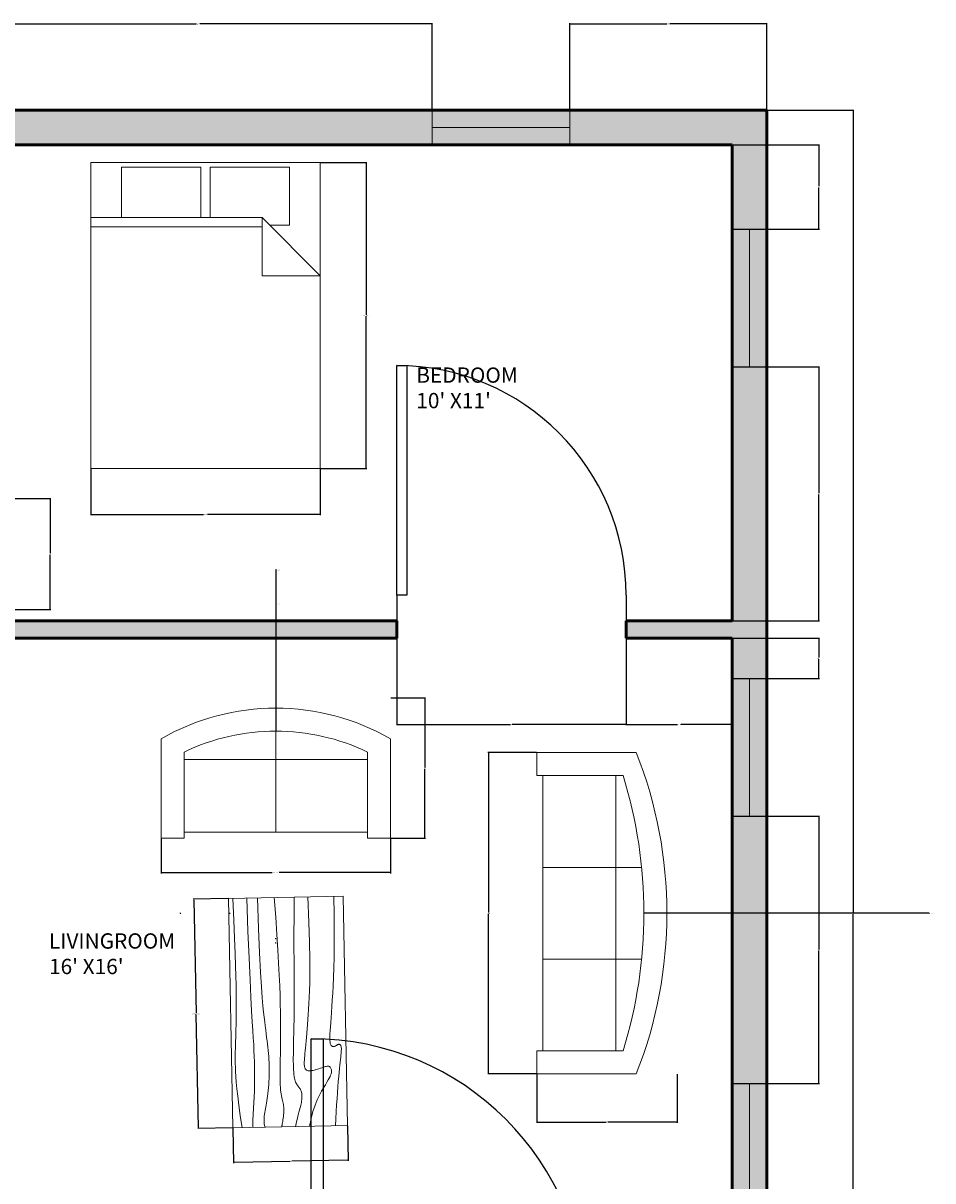
# Model space of a CAD drawing. Units: inches. Extents: x 7 to 493, y -11 to 454.
# Tile 4 of 4: x 255 to 493, y 152 to 454. Entities that reach past the tile are written whole.
import ezdxf

# ---------------------------------------------------------------- set-up
doc = ezdxf.new("R2010")
doc.units = ezdxf.units.IN
doc.header["$MEASUREMENT"] = 0
for name, color, linetype, lineweight in [('A-ANNO-DIMS', 2, 'Continuous', 18), ('A-AREA-IDEN', 7, 'Continuous', 25), ('A-WALL', 7, 'Continuous', 50), ('doors', 40, 'Continuous', 25), ('furniture', 220, 'Continuous', 18), ('window', 30, 'Continuous', 18)]:
    doc.layers.add(name, color=color, linetype=linetype, lineweight=lineweight)
doc.layers.add('A-WALL-PATT', color=251, linetype='Continuous', lineweight=13, true_color=0x636466)
doc.styles.get("Standard").update_dxf_attribs({"font": 'arial.ttf'})
doc.dimstyles.get("Standard").update_dxf_attribs({"dimtxt": 0.18, "dimasz": 0.18, "dimexe": 0.18, "dimexo": 0.0625, "dimgap": 0.09, "dimtad": 0, "dimtih": 1, "dimtoh": 1, "dimdec": 4, "dimzin": 0, "dimdsep": 46, "dimtxsty": 'Standard', "dimcen": 0.09, "dimadec": 0, "dimazin": 0, "dimtfac": 1, "dimtdec": 4, "dimtofl": 0, "dimtmove": 0, "dimatfit": 3, "dimfxl": 1, "dimtolj": 1, "dimtzin": 0, "dimarcsym": 0})

# ---------------------------------------------------------------- blocks, each defined once
blk = doc.blocks.new('Sofa - Roundback 7 ft.')
for p, q in [((-12.00002, -32.4421), (-12.00003, -6.5971)), ((11.99997, -32.4421), (11.99998, -6.5971)), ((-36.000027, -34), (-36.000027, -11.4696)), ((35.99998, -34), (35.99998, -11.4696)), ((-35.999844, -13.3819), (35.9998, -13.3819)), ((-36.000027, -32.4421), (35.99998, -32.4421))]:
    blk.add_line(p, q)
for points in [[(-36.000027, -34), (-42.000027, -34), (-42.000027, -8)], [(41.99998, -8), (41.99998, -34), (35.99998, -34)]]:
    blk.add_lwpolyline(points)
for centre, radius, start, end in [((0, -114.25), 114.25, 68.43141, 111.5686), ((-0.00001, -127.1968), 121.1968, 72.72033, 107.2797)]:
    blk.add_arc(centre, radius, start, end)
blk = doc.blocks.new('Sofa - Roundback Loveseat 5 ft.')
for p, q in [((0, -32.44198), (0, -5.99998)), ((-24, -33.99998), (-24, -11.46958)), ((24.00004, -33.99998), (24.00004, -11.46958)), ((-23.9998, -13.38178), (23.99986, -13.38178)), ((-24, -32.44198), (24.00004, -32.44198))]:
    blk.add_line(p, q)
for points in [[(-24, -33.99998), (-30, -33.99998), (-30, -7.99998)], [(30.00004, -7.99998), (30.00004, -33.99998), (24.00004, -33.99998)]]:
    blk.add_lwpolyline(points)
for centre, radius, start, end in [((0, -60.24998), 60.24998, 60.13715, 119.8628), ((0, -61.38438), 55.38444, 64.32083, 115.6792)]:
    blk.add_arc(centre, radius, start, end)
blk = doc.blocks.new('Bed - Queen')
for p, q in [((0, -80.00003), (0, 0)), ((0, 0), (59.99999, 0)), ((59.99999, 0), (59.99999, -80.00003)), ((7.99999, -1.2), (28.79998, -1.2)), ((7.99999, -14.4), (7.99999, -1.2)), ((28.79998, -1.2), (28.79998, -14.4)), ((31.19999, -1.2), (51.99999, -1.2)), ((31.19999, -14.4), (31.19999, -1.2)), ((51.99999, -1.2), (51.99999, -16.4)), ((0, -14.4), (44.8, -14.4)), ((59.99999, -29.6), (44.8, -14.4)), ((44.8, -14.4), (44.8, -29.6)), ((44.8, -16.8), (0, -16.8)), ((51.99999, -16.4), (46.79936, -16.4)), ((44.8, -29.6), (59.99999, -29.6)), ((59.99999, -80.00003), (0, -80.00003))]:
    blk.add_line(p, q)
blk = doc.blocks.new('Table - Rectangular Woodgrain 60 x 30 in.')
for p, q in [((0, 0), (0, -30)), ((60, 0), (0, 0)), ((60, -30), (60, 0)), ((0, -30), (60, -30))]:
    blk.add_line(p, q)
for points in [[(0, -2.4), (4.8155, -2.418), (9.0302, -2.4688), (12.709, -2.5477), (15.9167, -2.65), (18.7181, -2.7711), (21.1781, -2.9063), (23.3616, -3.0508), (25.3333, -3.2), (27.1477, -3.3495), (28.8172, -3.4958), (30.3437, -3.636), (31.7291, -3.7667), (32.9756, -3.8849), (34.0849, -3.9875), (35.059, -4.0714), (35.9, -4.1334), (36.6114, -4.1711), (37.2041, -4.1854), (37.6906, -4.1779), (38.0833, -4.15), (38.3948, -4.1034), (38.6375, -4.0396), (38.8239, -3.9602), (38.9666, -3.8667), (39.0764, -3.7608), (39.1573, -3.6448), (39.2116, -3.521), (39.2416, -3.3917), (39.2498, -3.2593), (39.2385, -3.1261), (39.21, -2.9944), (39.1666, -2.8667), (39.111, -2.7447), (39.0468, -2.6281), (38.978, -2.5163), (38.9083, -2.4083), (38.8418, -2.3035), (38.7823, -2.201), (38.7337, -2.1001), (38.7, -2), (38.6844, -1.9003), (38.6875, -1.8021), (38.7094, -1.707), (38.75, -1.6167), (38.8094, -1.5326), (38.8875, -1.4563), (38.9844, -1.3893), (39.1, -1.3333), (39.2351, -1.2896), (39.3937, -1.2583), (39.5804, -1.2396), (39.8, -1.2333), (40.057, -1.2396), (40.3562, -1.2583), (40.7023, -1.2896), (41.1, -1.3333), (41.5547, -1.3895), (42.0755, -1.4573), (42.6721, -1.5361), (43.3542, -1.625), (44.1316, -1.7233), (45.014, -1.8302), (46.0114, -1.9449), (47.1333, -2.0667), (48.3862, -2.1947), (49.7625, -2.3281), (51.2513, -2.4663), (52.8416, -2.6083), (54.5226, -2.7535), (56.2833, -2.9011), (58.1127, -3.0501), (60, -3.2)], [(0, -9.2), (6.5759, -9.0858), (11.9385, -9.0365), (16.2527, -9.0418), (19.6833, -9.0917), (22.3952, -9.1759), (24.5531, -9.2844), (26.322, -9.4069), (27.8666, -9.5333), (29.3241, -9.6553), (30.7203, -9.7719), (32.0532, -9.8837), (33.3208, -9.9917), (34.5213, -10.0965), (35.6526, -10.199), (36.7128, -10.2999), (37.7, -10.4), (38.6129, -10.4996), (39.4531, -10.5969), (40.223, -10.6895), (40.925, -10.775), (41.5613, -10.8512), (42.1344, -10.9156), (42.6465, -10.966), (43.1, -11), (43.4976, -11.0158), (43.8437, -11.0136), (44.143, -10.9942), (44.4, -10.9583), (44.6195, -10.9069), (44.8062, -10.8406), (44.9648, -10.7603), (45.1, -10.6667), (45.2155, -10.5598), (45.3114, -10.4365), (45.3871, -10.2929), (45.4416, -10.125), (45.4743, -9.929), (45.4844, -9.7011), (45.4709, -9.4371), (45.4333, -9.1333), (45.3716, -8.7883), (45.2896, -8.4104), (45.1919, -8.0107), (45.0833, -7.6), (44.9685, -7.1893), (44.8521, -6.7896), (44.7388, -6.4117), (44.6333, -6.0667), (44.54, -5.7628), (44.4614, -5.4979), (44.4001, -5.2675), (44.3583, -5.0667), (44.3384, -4.8909), (44.3427, -4.7354), (44.3736, -4.5956), (44.4333, -4.4667), (44.5236, -4.3453), (44.6427, -4.2333), (44.7884, -4.1339), (44.9583, -4.05), (45.1501, -3.9849), (45.3614, -3.9417), (45.59, -3.9234), (45.8333, -3.9333), (46.0915, -3.9749), (46.3734, -4.0531), (46.6906, -4.1736), (47.0542, -4.3417), (47.4756, -4.5629), (47.9661, -4.8427), (48.5372, -5.1866), (49.2, -5.6), (49.9676, -6.0844), (50.8594, -6.625), (51.8965, -7.2031), (53.1, -7.8), (54.491, -8.3969), (56.0906, -8.975), (57.9199, -9.5156), (60, -10)], [(0, -12.8), (5.1847, -12.9322), (9.6213, -13.0323), (13.3963, -13.1059), (16.5958, -13.1583), (19.3063, -13.1952), (21.614, -13.2219), (23.6054, -13.2439), (25.3666, -13.2667), (26.9728, -13.2947), (28.4531, -13.3281), (29.8256, -13.3663), (31.1083, -13.4083), (32.3191, -13.4535), (33.476, -13.501), (34.597, -13.5501), (35.7, -13.6), (36.7984, -13.6497), (37.8875, -13.6979), (38.9578, -13.743), (40, -13.7833), (41.0047, -13.8174), (41.9625, -13.8438), (42.864, -13.8607), (43.7, -13.8667), (44.4631, -13.8604), (45.1552, -13.8417), (45.7801, -13.8104), (46.3416, -13.7667), (46.8439, -13.7104), (47.2906, -13.6417), (47.6858, -13.5604), (48.0333, -13.4667), (48.3375, -13.3608), (48.6042, -13.2448), (48.8396, -13.121), (49.05, -12.9917), (49.2417, -12.8593), (49.4208, -12.7261), (49.5937, -12.5944), (49.7667, -12.4667), (49.9452, -12.3451), (50.1323, -12.2313), (50.3303, -12.1268), (50.5416, -12.0333), (50.7686, -11.9524), (51.0135, -11.8854), (51.2788, -11.8341), (51.5666, -11.8), (51.8785, -11.7843), (52.2116, -11.7865), (52.562, -11.8059), (52.926, -11.8417), (53.2998, -11.8931), (53.6795, -11.9594), (54.0614, -12.0397), (54.4416, -12.1333), (54.8223, -12.2401), (55.2293, -12.3625), (55.6942, -12.5037), (56.2489, -12.6667), (56.9251, -12.8547), (57.7545, -13.0708), (58.7689, -13.3182), (60, -13.6)], [(0, -18), (5.124, -17.7273), (9.6609, -17.5057), (13.6705, -17.3303), (17.2125, -17.1958), (20.3467, -17.0973), (23.1328, -17.0297), (25.6307, -16.9878), (27.9, -16.9667), (29.9928, -16.9617), (31.9302, -16.9703), (33.7254, -16.9907), (35.3917, -17.0208), (36.9423, -17.0588), (38.3906, -17.1026), (39.7499, -17.1503), (41.0333, -17.2), (42.2519, -17.2496), (43.4073, -17.2969), (44.4986, -17.3395), (45.525, -17.375), (46.4858, -17.4012), (47.3802, -17.4156), (48.2074, -17.416), (48.9667, -17.4), (49.6583, -17.3662), (50.2872, -17.3167), (50.8595, -17.2547), (51.3812, -17.1833), (51.8584, -17.1057), (52.2971, -17.025), (52.7034, -16.9443), (53.0833, -16.8667), (53.443, -16.7951), (53.789, -16.7313), (54.128, -16.6768), (54.4666, -16.6334), (54.8115, -16.6024), (55.1693, -16.5854), (55.5465, -16.5841), (55.95, -16.6), (56.3828, -16.6337), (56.8346, -16.6823), (57.2915, -16.7418), (57.7396, -16.8084), (58.165, -16.878), (58.5539, -16.9469), (58.8924, -17.0111), (59.1666, -17.0667), (59.3679, -17.1107), (59.5078, -17.1438), (59.6032, -17.1675), (59.6708, -17.1833), (59.7275, -17.193), (59.7901, -17.1979), (59.8753, -17.1998), (60, -17.2)], [(0, -22.4), (8.0098, -22.2501), (14.4094, -22.1011), (19.4168, -21.9535), (23.25, -21.8083), (26.1269, -21.6663), (28.2656, -21.5281), (29.884, -21.3947), (31.2, -21.2667), (32.3967, -21.1448), (33.5172, -21.0292), (34.5697, -20.9198), (35.5625, -20.8167), (36.5037, -20.7198), (37.4015, -20.6292), (38.2642, -20.5448), (39.1, -20.4667), (39.9164, -20.3951), (40.7187, -20.3313), (41.5117, -20.2768), (42.3, -20.2333), (43.0883, -20.2024), (43.8812, -20.1854), (44.6836, -20.1841), (45.5, -20.2), (46.3328, -20.234), (47.1747, -20.2844), (48.0163, -20.3488), (48.8479, -20.425), (49.66, -20.5106), (50.4429, -20.6031), (51.1872, -20.7004), (51.8833, -20.8), (52.5246, -20.8999), (53.1166, -20.9995), (53.6681, -21.0983), (54.1875, -21.1958), (54.6834, -21.2919), (55.1646, -21.3859), (55.6394, -21.4777), (56.1167, -21.5667), (56.6028, -21.6515), (57.0961, -21.7266), (57.5929, -21.7852), (58.0896, -21.8208), (58.5823, -21.8268), (59.0674, -21.7964), (59.5412, -21.723), (60, -21.6)], [(0, -25.2), (8.6355, -25.0504), (15.7026, -24.9031), (21.4049, -24.7606), (25.9458, -24.625), (29.529, -24.4988), (32.3578, -24.3844), (34.6359, -24.284), (36.5667, -24.2), (38.3213, -24.1341), (39.9417, -24.0854), (41.437, -24.0523), (42.8167, -24.0333), (44.0901, -24.0268), (45.2667, -24.0313), (46.3557, -24.0451), (47.3667, -24.0667), (48.309, -24.0947), (49.1928, -24.1287), (50.0284, -24.168), (50.826, -24.2125), (51.5959, -24.2617), (52.3483, -24.3151), (53.0935, -24.3725), (53.8417, -24.4334), (54.6009, -24.497), (55.3699, -24.561), (56.1454, -24.6226), (56.9239, -24.6792), (57.7021, -24.7279), (58.4764, -24.7662), (59.2435, -24.7911), (60, -24.8)], [(0, -28.8), (5.6867, -28.6681), (10.45, -28.5698), (14.407, -28.5012), (17.675, -28.4584), (20.3711, -28.4374), (22.6125, -28.4344), (24.5164, -28.4455), (26.2, -28.4667), (27.762, -28.4947), (29.2276, -28.5281), (30.6033, -28.5663), (31.8958, -28.6084), (33.1118, -28.6535), (34.2578, -28.7011), (35.3405, -28.7501), (36.3666, -28.8), (37.3443, -28.8497), (38.288, -28.8974), (39.2137, -28.9412), (40.1375, -28.9792), (41.0753, -29.0093), (42.0432, -29.0297), (43.0572, -29.0384), (44.1333, -29.0333), (45.2936, -29.0114), (46.5843, -28.9641), (48.0579, -28.8816), (49.7666, -28.7542), (51.7629, -28.5721), (54.0989, -28.3255), (56.8272, -28.0048), (60, -27.6)]]:
    blk.add_lwpolyline(points)
blk = doc.blocks.new('*U4')
for p, q in [((0, 0), (0, -6)), ((40, 0), (40, -6))]:
    blk.add_line(p, q)
blk.add_lwpolyline([(0, 0), (0, 40), (1.75, 40), (1.75, 0)], close=True)
blk.add_arc((0, 0), 40, 0, 90)
blk = doc.blocks.new('WIN-36IN')
for p, q in [((0, 0), (0, 9)), ((0, 9), (36, 9)), ((36, 9), (36, 0)), ((36, 9), (36, 4.5)), ((36, 4.5), (0, 4.5)), ((36, 0), (0, 0))]:
    blk.add_line(p, q)
blk = doc.blocks.new('*D12')
at = {"layer": 'A-ANNO-DIMS', "color": 0, "lineweight": -2, "transparency": 16777216}
for p, q in [((333.11, 417.82), (345.22, 417.82)), ((345.04, 417.64), (345.04, 378.01)), ((345.04, 338), (345.04, 377.63)), ((333.11, 337.82), (345.22, 337.82))]:
    blk.add_line(p, q, dxfattribs=at)
at = {"layer": 'A-ANNO-DIMS', "color": 0, "transparency": 16777216}
for points in [[(345.01, 417.64), (345.07, 417.64), (345.04, 417.82)], [(345.01, 338), (345.07, 338), (345.04, 337.82)]]:
    blk.add_solid(points, dxfattribs=at)
at = {"layer": 'Defpoints', "color": 0, "transparency": 16777216}
for p in [(333.04, 417.82), (345.04, 417.82), (333.04, 337.82)]:
    blk.add_point(p, dxfattribs=at)
at = {"layer": 'A-ANNO-DIMS', "color": 0, "transparency": 16777216, "insert": (345.04, 377.82), "char_height": 0.18, "attachment_point": 5}
blk.add_mtext('\\A1;QUEEN BED 80 TYP.', dxfattribs=at)
blk = doc.blocks.new('*D13')
at = {"layer": 'A-ANNO-DIMS', "color": 0, "lineweight": -2, "transparency": 16777216}
for p, q in [((273.04, 337.76), (273.04, 325.64)), ((333.04, 337.76), (333.04, 325.64)), ((273.22, 325.82), (302.51, 325.82)), ((332.86, 325.82), (303.57, 325.82))]:
    blk.add_line(p, q, dxfattribs=at)
at = {"layer": 'A-ANNO-DIMS', "color": 0, "transparency": 16777216}
for points in [[(273.22, 325.85), (273.22, 325.79), (273.04, 325.82)], [(332.86, 325.85), (332.86, 325.79), (333.04, 325.82)]]:
    blk.add_solid(points, dxfattribs=at)
at = {"layer": 'Defpoints', "color": 0, "transparency": 16777216}
for p in [(273.04, 337.82), (333.04, 337.82), (333.04, 325.82)]:
    blk.add_point(p, dxfattribs=at)
at = {"layer": 'A-ANNO-DIMS', "color": 0, "transparency": 16777216, "insert": (303.04, 325.82), "char_height": 0.18, "attachment_point": 5}
blk.add_mtext('\\A1;60 TYP.', dxfattribs=at)
blk = doc.blocks.new('*D14')
at = {"layer": 'A-ANNO-DIMS', "color": 0, "lineweight": -2, "transparency": 16777216}
for p, q in [((389.64, 263.58), (376.92, 263.58)), ((377.1, 263.4), (377.1, 221.76)), ((377.1, 179.76), (377.1, 221.4)), ((389.64, 179.58), (376.92, 179.58))]:
    blk.add_line(p, q, dxfattribs=at)
at = {"layer": 'A-ANNO-DIMS', "color": 0, "transparency": 16777216}
for points in [[(377.07, 263.4), (377.13, 263.4), (377.1, 263.58)], [(377.07, 179.76), (377.13, 179.76), (377.1, 179.58)]]:
    blk.add_solid(points, dxfattribs=at)
at = {"layer": 'Defpoints', "color": 0, "transparency": 16777216}
for p in [(389.7, 263.58), (377.1, 179.58), (389.7, 179.58)]:
    blk.add_point(p, dxfattribs=at)
at = {"layer": 'A-ANNO-DIMS', "color": 0, "transparency": 16777216, "insert": (377.1, 221.58), "char_height": 0.18, "attachment_point": 5}
blk.add_mtext('\\A1;SOFA 84', dxfattribs=at)
blk = doc.blocks.new('*D15')
at = {"layer": 'A-ANNO-DIMS', "color": 0, "lineweight": -2, "transparency": 16777216}
for p, q in [((389.7, 179.52), (389.7, 166.8)), ((426.37, 179.52), (426.37, 166.8)), ((389.88, 166.98), (407.82, 166.98)), ((426.19, 166.98), (408.26, 166.98))]:
    blk.add_line(p, q, dxfattribs=at)
at = {"layer": 'A-ANNO-DIMS', "color": 0, "transparency": 16777216}
for points in [[(389.88, 167.01), (389.88, 166.95), (389.7, 166.98)], [(426.19, 167.01), (426.19, 166.95), (426.37, 166.98)]]:
    blk.add_solid(points, dxfattribs=at)
at = {"layer": 'Defpoints', "color": 0, "transparency": 16777216}
for p in [(389.7, 179.58), (426.37, 179.58), (426.37, 166.98)]:
    blk.add_point(p, dxfattribs=at)
at = {"layer": 'A-ANNO-DIMS', "color": 0, "transparency": 16777216, "insert": (408.04, 166.98), "char_height": 0.18, "attachment_point": 5}
blk.add_mtext('\\A1;37', dxfattribs=at)
blk = doc.blocks.new('*D16')
at = {"layer": 'A-ANNO-DIMS', "color": 0, "lineweight": -2, "transparency": 16777216}
for p, q in [((291.43, 241.13), (291.43, 232.01)), ((351.43, 241.13), (351.43, 232.01)), ((291.61, 232.19), (320.52, 232.19)), ((351.25, 232.19), (322.34, 232.19))]:
    blk.add_line(p, q, dxfattribs=at)
at = {"layer": 'A-ANNO-DIMS', "color": 0, "transparency": 16777216}
for points in [[(291.61, 232.22), (291.61, 232.16), (291.43, 232.19)], [(351.25, 232.22), (351.25, 232.16), (351.43, 232.19)]]:
    blk.add_solid(points, dxfattribs=at)
at = {"layer": 'Defpoints', "color": 0, "transparency": 16777216}
for p in [(291.43, 241.19), (351.43, 241.19), (351.43, 232.19)]:
    blk.add_point(p, dxfattribs=at)
at = {"layer": 'A-ANNO-DIMS', "color": 0, "transparency": 16777216, "insert": (321.43, 232.19), "char_height": 0.18, "attachment_point": 5}
blk.add_mtext('\\A1;LOVESEAT 60', dxfattribs=at)
blk = doc.blocks.new('*D17')
at = {"layer": 'A-ANNO-DIMS', "color": 0, "lineweight": -2, "transparency": 16777216}
for p, q in [((351.49, 277.86), (360.61, 277.86)), ((360.43, 277.68), (360.43, 259.71)), ((360.43, 241.37), (360.43, 259.34)), ((351.49, 241.19), (360.61, 241.19))]:
    blk.add_line(p, q, dxfattribs=at)
at = {"layer": 'A-ANNO-DIMS', "color": 0, "transparency": 16777216}
for points in [[(360.4, 277.68), (360.46, 277.68), (360.43, 277.86)], [(360.4, 241.37), (360.46, 241.37), (360.43, 241.19)]]:
    blk.add_solid(points, dxfattribs=at)
at = {"layer": 'Defpoints', "color": 0, "transparency": 16777216}
for p in [(351.43, 277.86), (360.43, 277.86), (351.43, 241.19)]:
    blk.add_point(p, dxfattribs=at)
at = {"layer": 'A-ANNO-DIMS', "color": 0, "transparency": 16777216, "insert": (360.43, 259.52), "char_height": 0.18, "attachment_point": 5}
blk.add_mtext('\\A1;37', dxfattribs=at)
blk = doc.blocks.new('*D18')
at = {"layer": 'A-ANNO-DIMS', "color": 0, "lineweight": -2, "transparency": 16777216}
for p, q in [((308.97, 225.45), (299.85, 225.27)), ((300.04, 225.09), (300.62, 195.46)), ((301.22, 165.46), (300.63, 195.09)), ((310.16, 165.46), (301.04, 165.28))]:
    blk.add_line(p, q, dxfattribs=at)
at = {"layer": 'A-ANNO-DIMS', "color": 0, "transparency": 16777216}
for points in [[(300.07, 225.09), (300.01, 225.09), (300.03, 225.27)], [(301.25, 165.46), (301.19, 165.46), (301.22, 165.28)]]:
    blk.add_solid(points, dxfattribs=at)
at = {"layer": 'Defpoints', "color": 0, "transparency": 16777216}
for p in [(309.03, 225.45), (301.22, 165.28), (310.22, 165.46)]:
    blk.add_point(p, dxfattribs=at)
at = {"layer": 'A-ANNO-DIMS', "color": 0, "transparency": 16777216, "insert": (300.63, 195.28), "char_height": 0.18, "attachment_point": 5}
blk.add_mtext('\\A1;COFFEE TABLE 60', dxfattribs=at)
blk = doc.blocks.new('*D19')
at = {"layer": 'A-ANNO-DIMS', "color": 0, "lineweight": -2, "transparency": 16777216}
for p, q in [((310.22, 165.4), (310.4, 156.28)), ((340.21, 165.99), (340.39, 156.88)), ((310.58, 156.47), (325.17, 156.75)), ((340.21, 157.05), (325.61, 156.76))]:
    blk.add_line(p, q, dxfattribs=at)
at = {"layer": 'A-ANNO-DIMS', "color": 0, "transparency": 16777216}
for points in [[(310.57, 156.5), (310.58, 156.44), (310.4, 156.46)], [(340.21, 157.08), (340.21, 157.02), (340.39, 157.06)]]:
    blk.add_solid(points, dxfattribs=at)
at = {"layer": 'Defpoints', "color": 0, "transparency": 16777216}
for p in [(310.22, 165.46), (340.21, 166.05), (340.39, 157.06)]:
    blk.add_point(p, dxfattribs=at)
at = {"layer": 'A-ANNO-DIMS', "color": 0, "transparency": 16777216, "insert": (325.39, 156.76), "char_height": 0.18, "attachment_point": 5}
blk.add_mtext('\\A1;30', dxfattribs=at)
blk = doc.blocks.new('*D23')
at = {"layer": 'A-ANNO-DIMS', "color": 0, "lineweight": -2, "transparency": 16777216}
for p, q in [((449.87, 431.49), (472.59, 431.49)), ((472.41, 431.31), (472.41, 221.67)), ((472.41, 11.67), (472.41, 221.3)), ((449.87, 11.49), (472.59, 11.49))]:
    blk.add_line(p, q, dxfattribs=at)
at = {"layer": 'A-ANNO-DIMS', "color": 0, "transparency": 16777216}
for points in [[(472.38, 431.31), (472.44, 431.31), (472.41, 431.49)], [(472.38, 11.67), (472.44, 11.67), (472.41, 11.49)]]:
    blk.add_solid(points, dxfattribs=at)
at = {"layer": 'Defpoints', "color": 0, "transparency": 16777216}
for p in [(449.81, 431.49), (472.41, 431.49), (449.81, 11.49)]:
    blk.add_point(p, dxfattribs=at)
at = {"layer": 'A-ANNO-DIMS', "color": 0, "transparency": 16777216, "insert": (472.41, 221.49), "char_height": 0.18, "attachment_point": 5}
blk.add_mtext('\\A1;420', dxfattribs=at)
blk = doc.blocks.new('*D28')
at = {"layer": 'A-ANNO-DIMS', "color": 0, "lineweight": -2, "transparency": 16777216}
for p, q in [((239.81, 422.55), (239.81, 454.27)), ((239.99, 454.09), (300.63, 454.09)), ((362.18, 454.09), (301.54, 454.09)), ((362.36, 431.55), (362.36, 454.27))]:
    blk.add_line(p, q, dxfattribs=at)
at = {"layer": 'A-ANNO-DIMS', "color": 0, "transparency": 16777216}
for points in [[(239.99, 454.12), (239.99, 454.06), (239.81, 454.09)], [(362.18, 454.12), (362.18, 454.06), (362.36, 454.09)]]:
    blk.add_solid(points, dxfattribs=at)
at = {"layer": 'Defpoints', "color": 0, "transparency": 16777216}
for p in [(362.36, 454.09), (362.36, 431.49), (239.81, 422.49)]:
    blk.add_point(p, dxfattribs=at)
at = {"layer": 'A-ANNO-DIMS', "color": 0, "transparency": 16777216, "insert": (301.08, 454.09), "char_height": 0.18, "attachment_point": 5}
blk.add_mtext('\\A1;122.55', dxfattribs=at)
blk = doc.blocks.new('*D29')
at = {"layer": 'A-ANNO-DIMS', "color": 0, "lineweight": -2, "transparency": 16777216}
for p, q in [((398.36, 431.55), (398.36, 454.27)), ((398.54, 454.09), (423.69, 454.09)), ((449.63, 454.09), (424.48, 454.09)), ((449.81, 431.55), (449.81, 454.27))]:
    blk.add_line(p, q, dxfattribs=at)
at = {"layer": 'A-ANNO-DIMS', "color": 0, "transparency": 16777216}
for points in [[(398.54, 454.12), (398.54, 454.06), (398.36, 454.09)], [(449.63, 454.12), (449.63, 454.06), (449.81, 454.09)]]:
    blk.add_solid(points, dxfattribs=at)
at = {"layer": 'Defpoints', "color": 0, "transparency": 16777216}
for p in [(449.81, 454.09), (398.36, 431.49), (449.81, 431.49)]:
    blk.add_point(p, dxfattribs=at)
at = {"layer": 'A-ANNO-DIMS', "color": 0, "transparency": 16777216, "insert": (424.08, 454.09), "char_height": 0.18, "attachment_point": 5}
blk.add_mtext('\\A1;51.45', dxfattribs=at)
blk = doc.blocks.new('*D39')
at = {"layer": 'A-ANNO-DIMS', "color": 0, "lineweight": -2, "transparency": 16777216}
for p, q in [((440.87, 246.95), (463.59, 246.95)), ((463.41, 246.77), (463.41, 212.21)), ((463.41, 177.29), (463.41, 211.85)), ((440.87, 177.11), (463.59, 177.11))]:
    blk.add_line(p, q, dxfattribs=at)
at = {"layer": 'A-ANNO-DIMS', "color": 0, "transparency": 16777216}
for points in [[(463.38, 246.77), (463.44, 246.77), (463.41, 246.95)], [(463.38, 177.29), (463.44, 177.29), (463.41, 177.11)]]:
    blk.add_solid(points, dxfattribs=at)
at = {"layer": 'Defpoints', "color": 0, "transparency": 16777216}
for p in [(440.81, 246.95), (440.81, 177.11), (463.41, 177.11)]:
    blk.add_point(p, dxfattribs=at)
at = {"layer": 'A-ANNO-DIMS', "color": 0, "transparency": 16777216, "insert": (463.41, 212.03), "char_height": 0.18, "attachment_point": 5}
blk.add_mtext('\\A1;69.83', dxfattribs=at)
blk = doc.blocks.new('*D40')
at = {"layer": 'A-ANNO-DIMS', "color": 0, "lineweight": -2, "transparency": 16777216}
for p, q in [((440.87, 293.49), (463.59, 293.49)), ((463.41, 293.31), (463.41, 288.4)), ((463.41, 283.13), (463.41, 288.03)), ((440.87, 282.95), (463.59, 282.95))]:
    blk.add_line(p, q, dxfattribs=at)
at = {"layer": 'A-ANNO-DIMS', "color": 0, "transparency": 16777216}
for points in [[(463.38, 293.31), (463.44, 293.31), (463.41, 293.49)], [(463.38, 283.13), (463.44, 283.13), (463.41, 282.95)]]:
    blk.add_solid(points, dxfattribs=at)
at = {"layer": 'Defpoints', "color": 0, "transparency": 16777216}
for p in [(440.81, 293.49), (440.81, 282.95), (463.41, 282.95)]:
    blk.add_point(p, dxfattribs=at)
at = {"layer": 'A-ANNO-DIMS', "color": 0, "transparency": 16777216, "insert": (463.41, 288.22), "char_height": 0.18, "attachment_point": 5}
blk.add_mtext('\\A1;10.54', dxfattribs=at)
blk = doc.blocks.new('*D41')
at = {"layer": 'A-ANNO-DIMS', "color": 0, "lineweight": -2, "transparency": 16777216}
for p, q in [((440.87, 364.41), (463.59, 364.41)), ((463.41, 364.23), (463.41, 331.38)), ((463.41, 298.17), (463.41, 331.02)), ((440.87, 297.99), (463.59, 297.99))]:
    blk.add_line(p, q, dxfattribs=at)
at = {"layer": 'A-ANNO-DIMS', "color": 0, "transparency": 16777216}
for points in [[(463.38, 364.23), (463.44, 364.23), (463.41, 364.41)], [(463.38, 298.17), (463.44, 298.17), (463.41, 297.99)]]:
    blk.add_solid(points, dxfattribs=at)
at = {"layer": 'Defpoints', "color": 0, "transparency": 16777216}
for p in [(440.81, 364.41), (440.81, 297.99), (463.41, 297.99)]:
    blk.add_point(p, dxfattribs=at)
at = {"layer": 'A-ANNO-DIMS', "color": 0, "transparency": 16777216, "insert": (463.41, 331.2), "char_height": 0.18, "attachment_point": 5}
blk.add_mtext('\\A1;66.43', dxfattribs=at)
blk = doc.blocks.new('*D42')
at = {"layer": 'A-ANNO-DIMS', "color": 0, "lineweight": -2, "transparency": 16777216}
for p, q in [((440.87, 422.49), (463.59, 422.49)), ((463.41, 422.31), (463.41, 411.63)), ((463.41, 400.59), (463.41, 411.27)), ((440.87, 400.41), (463.59, 400.41))]:
    blk.add_line(p, q, dxfattribs=at)
at = {"layer": 'A-ANNO-DIMS', "color": 0, "transparency": 16777216}
for points in [[(463.38, 422.31), (463.44, 422.31), (463.41, 422.49)], [(463.38, 400.59), (463.44, 400.59), (463.41, 400.41)]]:
    blk.add_solid(points, dxfattribs=at)
at = {"layer": 'Defpoints', "color": 0, "transparency": 16777216}
for p in [(440.81, 422.49), (440.81, 400.41), (463.41, 400.41)]:
    blk.add_point(p, dxfattribs=at)
at = {"layer": 'A-ANNO-DIMS', "color": 0, "transparency": 16777216, "insert": (463.41, 411.45), "char_height": 0.18, "attachment_point": 5}
blk.add_mtext('\\A1;22.07', dxfattribs=at)
blk = doc.blocks.new('*D53')
at = {"layer": 'A-ANNO-DIMS', "color": 0, "lineweight": -2, "transparency": 16777216}
for p, q in [((353.05, 293.42), (353.05, 270.71)), ((413.05, 293.42), (413.05, 270.71)), ((353.23, 270.89), (382.83, 270.89)), ((412.87, 270.89), (383.27, 270.89))]:
    blk.add_line(p, q, dxfattribs=at)
at = {"layer": 'A-ANNO-DIMS', "color": 0, "transparency": 16777216}
for points in [[(353.23, 270.92), (353.23, 270.86), (353.05, 270.89)], [(412.87, 270.92), (412.87, 270.86), (413.05, 270.89)]]:
    blk.add_solid(points, dxfattribs=at)
at = {"layer": 'Defpoints', "color": 0, "transparency": 16777216}
for p in [(353.05, 293.49), (413.05, 293.49), (353.05, 270.89)]:
    blk.add_point(p, dxfattribs=at)
at = {"layer": 'A-ANNO-DIMS', "color": 0, "transparency": 16777216, "insert": (383.05, 270.89), "char_height": 0.18, "attachment_point": 5}
blk.add_mtext('\\A1;60', dxfattribs=at)
blk = doc.blocks.new('*D54')
at = {"layer": 'A-ANNO-DIMS', "color": 0, "lineweight": -2, "transparency": 16777216}
for p, q in [((413.05, 293.42), (413.05, 270.71)), ((440.81, 293.42), (440.81, 270.71)), ((413.23, 270.89), (426.46, 270.89)), ((440.63, 270.89), (427.39, 270.89))]:
    blk.add_line(p, q, dxfattribs=at)
at = {"layer": 'A-ANNO-DIMS', "color": 0, "transparency": 16777216}
for points in [[(413.23, 270.92), (413.23, 270.86), (413.05, 270.89)], [(440.63, 270.92), (440.63, 270.86), (440.81, 270.89)]]:
    blk.add_solid(points, dxfattribs=at)
at = {"layer": 'Defpoints', "color": 0, "transparency": 16777216}
for p in [(413.05, 293.49), (440.81, 293.49), (413.05, 270.89)]:
    blk.add_point(p, dxfattribs=at)
at = {"layer": 'A-ANNO-DIMS', "color": 0, "transparency": 16777216, "insert": (426.93, 270.89), "char_height": 0.18, "attachment_point": 5}
blk.add_mtext('\\A1;27.754', dxfattribs=at)
blk = doc.blocks.new('*D55')
at = {"layer": 'A-ANNO-DIMS', "color": 0, "lineweight": -2, "transparency": 16777216}
for p, q in [((239.87, 329.99), (262.59, 329.99)), ((262.41, 329.81), (262.41, 315.67)), ((262.41, 301.17), (262.41, 315.3)), ((239.87, 300.99), (262.59, 300.99))]:
    blk.add_line(p, q, dxfattribs=at)
at = {"layer": 'A-ANNO-DIMS', "color": 0, "transparency": 16777216}
for points in [[(262.38, 329.81), (262.44, 329.81), (262.41, 329.99)], [(262.38, 301.17), (262.44, 301.17), (262.41, 300.99)]]:
    blk.add_solid(points, dxfattribs=at)
at = {"layer": 'Defpoints', "color": 0, "transparency": 16777216}
for p in [(239.81, 329.99), (239.81, 300.99), (262.41, 300.99)]:
    blk.add_point(p, dxfattribs=at)
at = {"layer": 'A-ANNO-DIMS', "color": 0, "transparency": 16777216, "insert": (262.41, 315.49), "char_height": 0.18, "attachment_point": 5}
blk.add_mtext('\\A1;29', dxfattribs=at)
blk = doc.blocks.new('*D59')
at = {"layer": 'A-ANNO-DIMS', "color": 0, "lineweight": -2, "transparency": 16777216}
for p, q in [((296.42, 221.58), (296.6, 221.58)), ((296.51, 221.49), (296.51, 221.67)), ((490.42, 221.58), (417.88, 221.58))]:
    blk.add_line(p, q, dxfattribs=at)
at = {"layer": 'A-ANNO-DIMS', "color": 0, "transparency": 16777216}
blk.add_solid([(417.88, 221.61), (417.88, 221.55), (417.7, 221.58)], dxfattribs=at)
at = {"layer": 'Defpoints', "color": 0, "transparency": 16777216}
for p in [(296.51, 221.58), (417.7, 221.58)]:
    blk.add_point(p, dxfattribs=at)
at = {"layer": 'A-ANNO-DIMS', "color": 0, "transparency": 16777216, "insert": (490.9, 221.58), "char_height": 0.18, "attachment_point": 5}
blk.add_mtext('\\A1;R121.2', dxfattribs=at)
blk = doc.blocks.new('*D60')
at = {"layer": 'A-ANNO-DIMS', "color": 0, "lineweight": -2, "transparency": 16777216}
for p, q in [((309.36, 221.58), (309.54, 221.58)), ((309.45, 221.49), (309.45, 221.67)), ((492.25, 221.58), (423.88, 221.58))]:
    blk.add_line(p, q, dxfattribs=at)
at = {"layer": 'A-ANNO-DIMS', "color": 0, "transparency": 16777216}
blk.add_solid([(423.88, 221.61), (423.88, 221.55), (423.7, 221.58)], dxfattribs=at)
at = {"layer": 'Defpoints', "color": 0, "transparency": 16777216}
for p in [(309.45, 221.58), (423.7, 221.58)]:
    blk.add_point(p, dxfattribs=at)
at = {"layer": 'A-ANNO-DIMS', "color": 0, "transparency": 16777216, "insert": (492.8, 221.58), "char_height": 0.18, "attachment_point": 5}
blk.add_mtext('\\A1;R114.25', dxfattribs=at)
blk = doc.blocks.new('*D61')
at = {"layer": 'A-ANNO-DIMS', "color": 0, "lineweight": -2, "transparency": 16777216}
for p, q in [((321.61, 311.34), (321.43, 311.34)), ((321.43, 311.34), (321.43, 275.37)), ((321.34, 214.94), (321.52, 214.94)), ((321.43, 214.85), (321.43, 215.03))]:
    blk.add_line(p, q, dxfattribs=at)
at = {"layer": 'A-ANNO-DIMS', "color": 0, "transparency": 16777216}
blk.add_solid([(321.4, 275.37), (321.46, 275.37), (321.43, 275.19)], dxfattribs=at)
at = {"layer": 'Defpoints', "color": 0, "transparency": 16777216}
for p in [(321.43, 275.19), (321.43, 214.94)]:
    blk.add_point(p, dxfattribs=at)
at = {"layer": 'A-ANNO-DIMS', "color": 0, "transparency": 16777216, "insert": (322.09, 311.34), "char_height": 0.18, "attachment_point": 5}
blk.add_mtext('\\A1;R60.25', dxfattribs=at)
blk = doc.blocks.new('*D62')
at = {"layer": 'A-ANNO-DIMS', "color": 0, "lineweight": -2, "transparency": 16777216}
for p, q in [((321.61, 302.42), (321.43, 302.42)), ((321.43, 302.42), (321.43, 269.37)), ((321.34, 213.81), (321.52, 213.81)), ((321.43, 213.72), (321.43, 213.9))]:
    blk.add_line(p, q, dxfattribs=at)
at = {"layer": 'A-ANNO-DIMS', "color": 0, "transparency": 16777216}
blk.add_solid([(321.4, 269.37), (321.46, 269.37), (321.43, 269.19)], dxfattribs=at)
at = {"layer": 'Defpoints', "color": 0, "transparency": 16777216}
for p in [(321.43, 269.19), (321.43, 213.81)]:
    blk.add_point(p, dxfattribs=at)
at = {"layer": 'A-ANNO-DIMS', "color": 0, "transparency": 16777216, "insert": (322.09, 302.42), "char_height": 0.18, "attachment_point": 5}
blk.add_mtext('\\A1;R55.38', dxfattribs=at)

msp = doc.modelspace()

# ---------------------------------------------------------------- hatches: boundary and pattern name
at = {"layer": 'A-WALL-PATT'}
h = msp.add_hatch(color=256, dxfattribs=at)
h.dxf.hatch_style = 1
h.paths.add_polyline_path([(29.8054, 11.4863), (449.8054, 11.4863), (449.8054, 431.4863), (29.8054, 431.4863)])
h.paths.add_polyline_path([(38.8054, 422.4863), (235.3054, 422.4863), (235.3054, 362.4863), (179.8054, 362.4863), (179.8054, 390.4863), (170.8054, 390.4863), (170.8054, 293.4863), (353.0513, 293.4863), (353.0513, 297.9863), (239.8054, 297.9863), (235.3054, 297.9863), (179.8054, 297.9863), (179.8054, 357.9863), (235.3054, 357.9863), (235.3054, 329.9863), (239.8054, 329.9863), (239.8054, 422.4863), (440.8054, 422.4863), (440.8054, 297.9863), (413.0513, 297.9863), (413.0513, 293.4863), (440.8054, 293.4863), (440.8054, 110.4863), (402.7135, 110.4863), (402.7135, 101.5532), (402.7135, 101.4863), (440.8054, 101.4863), (440.8054, 20.4863), (179.8054, 20.4863), (179.8054, 101.4863), (255.3658, 101.4863), (255.3658, 110.4863), (179.8054, 110.4863), (179.8054, 146.9794), (170.8054, 146.9794), (170.8054, 20.4863), (117.9037, 20.4863), (117.9037, 15.9863), (81.9037, 15.9863), (81.9037, 20.4863), (38.8054, 20.4863), (38.8054, 125.4863), (118.4942, 125.4863), (118.4942, 129.9863), (38.8054, 129.9863), (38.8054, 225.9863), (170.8054, 225.9863), (170.8054, 192.9161), (179.8054, 192.9161), (179.8054, 233.4863), (170.8054, 233.4863), (170.8054, 230.4863), (38.8054, 230.4863)], flags=16)
h.paths.add_polyline_path([(53.2938, 207.1427), (65.8095, 207.1427), (67.0594, 215.1427), (83.5282, 215.1427), (84.7782, 207.1427), (93.8095, 207.1427), (95.0594, 215.1427), (111.5282, 215.1427), (112.7782, 207.1427), (125.2938, 207.1427), (125.2938, 198.6271), (133.2938, 197.3771), (133.2938, 180.9083), (125.2938, 179.6583), (125.2938, 171.1427), (112.7782, 171.1427), (111.5282, 163.1427), (95.0594, 163.1427), (93.8095, 171.1427), (84.7782, 171.1427), (83.5282, 163.1427), (67.0594, 163.1427), (65.8095, 171.1427), (53.2938, 171.1427), (53.2938, 179.6583), (45.2938, 180.9083), (45.2938, 197.3771), (53.2938, 198.6271)], flags=0)
h.paths.add_polyline_path([(98.6154, 202.5867), (98.6833, 202.7415), (98.7209, 202.9031), (98.7311, 203.0686), (98.717, 203.2352), (98.6813, 203.3997), (98.6271, 203.5594), (98.5576, 203.7119), (98.4774, 203.8575), (98.3913, 203.9974), (98.2332, 204.2423), (98.1033, 204.4662), (98.0223, 204.7063), (98.0302, 204.9526), (98.1325, 205.1802), (98.329, 205.372), (98.3993, 205.406), (98.2782, 205.3224), (98.1805, 205.227), (98.1063, 205.1219), (98.0555, 205.0089), (98.0282, 204.8901), (98.0243, 204.7674), (98.0438, 204.6427), (98.086, 204.5175), (98.1467, 204.3914), (98.221, 204.2633), (98.3042, 204.1323), (98.4533, 203.9013), (98.6038, 203.6279), (98.7103, 203.3143), (98.7386, 202.9794), (98.6633, 202.6554)], flags=0)
h.paths.add_polyline_path([(67.2938, 216.6427), (83.2938, 216.6427), (83.45, 215.6427), (67.1375, 215.6427)], flags=0)
h.paths.add_polyline_path([(43.7938, 197.1427), (44.7938, 197.2989), (44.7938, 180.9864), (43.7938, 181.1427)], flags=0)
h.paths.add_polyline_path([(106.3833, 198.8302), (106.2808, 199.0177), (106.1587, 199.2052), (106.023, 199.3927), (105.8794, 199.5802), (105.6298, 199.9018), (105.4605, 200.1427), (105.3438, 200.33), (105.1938, 200.6147), (105.0892, 200.9776), (105.1, 201.3227), (105.1358, 201.3994), (105.0972, 201.2325), (105.0918, 201.0599), (105.1167, 200.8823), (105.169, 200.7008), (105.2456, 200.5164), (105.3438, 200.33), (105.4605, 200.1427), (105.5923, 199.9552), (105.7339, 199.7677), (105.8794, 199.5802), (106.1138, 199.2741), (106.3496, 198.9121)], flags=0)
h.paths.add_polyline_path([(124.5037, 189.2544), (124.6786, 189.213), (124.7978, 189.1834), (124.8824, 189.1635), (124.9532, 189.1515), (125.0583, 189.1432), (125.138, 189.143), (124.9529, 189.147), (124.7978, 189.1834), (124.5749, 189.2388)], flags=0)
h.paths.add_polyline_path([(95.2938, 216.6427), (111.2938, 216.6427), (111.45, 215.6427), (95.1375, 215.6427)], flags=0)
h.paths.add_polyline_path([(191.6785, 332.1221), (224.065, 332.1221), (224.065, 343.8649), (191.6785, 343.8649)], flags=8)
h.paths.add_polyline_path([(196.7522, 379.4931), (229.1387, 379.4931), (229.1387, 391.2359), (196.7522, 391.2359)], flags=8)
h.paths.add_polyline_path([(232.397, 56.3062), (260.115, 56.3062), (260.115, 68.0654), (232.397, 68.0654)], flags=8)
h.paths.add_polyline_path([(90.1783, 70.3293), (134.3492, 70.3293), (134.3492, 82.0885), (90.1783, 82.0885)], flags=8)
h.paths.add_polyline_path([(126.7274, 208.2711), (165.9297, 208.2711), (165.9297, 220.0303), (126.7274, 220.0303)], flags=8)
h.paths.add_polyline_path([(261.4741, 205.6105), (297.4786, 205.6105), (297.4786, 217.3697), (261.4741, 217.3697)], flags=8)
h.paths.add_polyline_path([(77.3838, 283.1969), (106.5561, 283.1969), (106.5561, 294.9561), (77.3838, 294.9561)], flags=8)
h.paths.add_polyline_path([(357.5163, 353.5423), (386.6886, 353.5423), (386.6886, 365.3015), (357.5163, 365.3015)], flags=8)

# ---------------------------------------------------------------- linework, layer by layer
at = {"layer": 'A-WALL'}
for p, q in [((239.8054, 422.4863), (440.8054, 422.4863)), ((440.8054, 422.4863), (440.8054, 297.9863)), ((239.8054, 297.9863), (353.0513, 297.9863)), ((353.0513, 293.4863), (353.0513, 297.9863)), ((413.0513, 297.9863), (440.8054, 297.9863)), ((413.0513, 297.9863), (413.0513, 293.4863)), ((170.8054, 293.4863), (353.0513, 293.4863)), ((413.0513, 293.4863), (440.8054, 293.4863)), ((440.8054, 293.4863), (440.8054, 110.4863))]:
    msp.add_line(p, q, dxfattribs=at)
msp.add_lwpolyline([(29.8054, 431.4863), (449.8054, 431.4863), (449.8054, 11.4863), (29.8054, 11.4863)], close=True, dxfattribs=at)

# ---------------------------------------------------------------- block references
at = {"layer": 'doors', "xscale": 1.5, "yscale": 1.5, "zscale": 1.5}
msp.add_blockref('*U4', (353.0513, 304.7363), dxfattribs=at)
at = {"layer": 'doors', "xscale": 1.799999418286923, "yscale": 1.799999418286923, "zscale": 1.799999418286923, "rotation": 0.026594711782106}
msp.add_blockref('*U4', (330.7085, 116.7863), dxfattribs=at)
at = {"layer": 'furniture'}
for name, p in [('Bed - Queen', (273.0433, 417.8223)), ('Sofa - Roundback Loveseat 5 ft.', (321.4299, 275.1898))]:
    msp.add_blockref(name, p, dxfattribs=at)
for name, p, rotation in [('Sofa - Roundback 7 ft.', (423.7035, 221.5787), 270), ('Table - Rectangular Woodgrain 60 x 30 in.', (339.0252, 226.0416), 271.1331455584855)]:
    msp.add_blockref(name, p, dxfattribs=dict(at, rotation=rotation))
at = {"layer": 'window'}
msp.add_blockref('WIN-36IN', (362.3581, 422.486), dxfattribs=at)
at = {"layer": 'window', "extrusion": (0, 0, -1), "zscale": -1, "rotation": 269.9999999999964}
for p in [(-449.8057, 400.4146), (-449.8057, 282.9467), (-449.8057, 177.1129)]:
    msp.add_blockref('WIN-36IN', p, dxfattribs=at)

# ---------------------------------------------------------------- texts
at = {"layer": 'A-AREA-IDEN', "char_height": 0.2, "attachment_point": 1}
for s, insert in [("{\\H20x;BEDROOM\\P10' X11'}", (358.1747, 364.2638)), ("{\\H20x;LIVINGROOM\\P16' X16'}", (262.1326, 216.332))]:
    msp.add_mtext_dynamic_manual_height_columns(s, width=58.591086, gutter_width=1, heights=[0], dxfattribs=dict(at, insert=insert))

# ---------------------------------------------------------------- dimensions: what is measured, and where the dimension line sits
at = {"layer": 'A-ANNO-DIMS'}
for base, p1, p2, override, picture, middle in [((362.3579, 454.0863), (239.8054, 422.4863), (362.3579, 431.4863), {"dimdec": 2, "dimlfac": 1, "dimrnd": 0, "dimzin": 0, "dimdsep": 46, "dimlunit": 2}, '*D28', (301.0816, 454.0863)), ((449.8054, 454.0863), (398.3579, 431.4863), (449.8054, 431.4863), {"dimdec": 2, "dimlfac": 1, "dimrnd": 0, "dimzin": 0, "dimdsep": 46, "dimlunit": 2}, '*D29', (424.0816, 454.0863)), ((426.3702, 166.9788), (389.7035, 179.5788), (426.3702, 179.5788), {"dimdec": 0, "dimlfac": 1, "dimrnd": 0, "dimzin": 0, "dimdsep": 46, "dimlunit": 2}, '*D15', (408.0369, 166.9788))]:
    dim = msp.add_linear_dim(base=base, p1=p1, p2=p2, dimstyle='Standard', override=override, dxfattribs=at)
    dim.commit()
    dim.dimension.update_dxf_attribs({"geometry": picture, "text_midpoint": middle})
for base, p1, p2, angle, override, picture, middle in [((472.4054, 431.4863), (449.8054, 11.4863), (449.8054, 431.4863), 90, {"dimdec": 0, "dimlfac": 1, "dimrnd": 0, "dimzin": 0, "dimdsep": 46, "dimlunit": 2}, '*D23', (472.4054, 221.4863)), ((463.4054, 400.4148), (440.8054, 422.4863), (440.8054, 400.4148), 270, {"dimdec": 2, "dimlfac": 1, "dimrnd": 0, "dimzin": 0, "dimdsep": 46, "dimlunit": 2}, '*D42', (463.4054, 411.4506)), ((463.4054, 297.9863), (440.8054, 364.4148), (440.8054, 297.9863), 270, {"dimdec": 2, "dimlfac": 1, "dimrnd": 0, "dimzin": 0, "dimdsep": 46, "dimlunit": 2}, '*D41', (463.4054, 331.2006)), ((262.4054, 300.9863), (239.8054, 329.9863), (239.8054, 300.9863), 270, {"dimdec": 0, "dimlfac": 1, "dimrnd": 0, "dimzin": 0, "dimdsep": 46, "dimlunit": 2}, '*D55', (262.4054, 315.4863)), ((353.0513, 270.8863), (413.0513, 293.4863), (353.0513, 293.4863), 180, {"dimdec": 0, "dimlfac": 1, "dimrnd": 0, "dimzin": 0, "dimdsep": 46, "dimlunit": 2}, '*D53', (383.0513, 270.8863)), ((413.0513, 270.8863), (440.8054, 293.4863), (413.0513, 293.4863), 180, {"dimdec": 3, "dimlfac": 1, "dimrnd": 0, "dimzin": 0, "dimdsep": 46, "dimlunit": 2}, '*D54', (426.9283, 270.8863)), ((463.4054, 282.9469), (440.8054, 293.4863), (440.8054, 282.9469), 270, {"dimdec": 2, "dimlfac": 1, "dimrnd": 0, "dimzin": 0, "dimdsep": 46, "dimlunit": 2}, '*D40', (463.4054, 288.2166)), ((360.43, 277.8565), (351.43, 241.1898), (351.43, 277.8565), 90, {"dimdec": 0, "dimlfac": 1, "dimrnd": 0, "dimzin": 0, "dimdsep": 46, "dimlunit": 2}, '*D17', (360.43, 259.5232)), ((463.4054, 177.1131), (440.8054, 246.9469), (440.8054, 177.1131), 270, {"dimdec": 2, "dimlfac": 1, "dimrnd": 0, "dimzin": 0, "dimdsep": 46, "dimlunit": 2}, '*D39', (463.4054, 212.03)), ((340.3897, 157.0551), (310.2176, 165.46), (340.2117, 166.0533), 1.133146, {"dimdec": 0, "dimlfac": 1, "dimrnd": 0, "dimzin": 0, "dimdsep": 46, "dimlunit": 2}, '*D19', (325.3927, 156.7584))]:
    dim = msp.add_linear_dim(base=base, p1=p1, p2=p2, angle=angle, dimstyle='Standard', override=override, dxfattribs=at)
    dim.commit()
    dim.dimension.update_dxf_attribs({"geometry": picture, "text_midpoint": middle})
for base, p1, p2, angle, text, picture, middle in [((345.0433, 417.8223), (333.0433, 337.8223), (333.0433, 417.8223), 90, 'QUEEN BED <> TYP.', '*D12', (345.0433, 377.8223)), ((377.1035, 179.5788), (389.7035, 263.5788), (389.7035, 179.5788), 270, 'SOFA <>', '*D14', (377.1035, 221.5788)), ((301.2194, 165.282), (309.0311, 225.4483), (310.2176, 165.46), 271.133146, 'COFFEE TABLE <>', '*D18', (300.6261, 195.2762))]:
    dim = msp.add_linear_dim(base=base, p1=p1, p2=p2, angle=angle, text=text, dimstyle='Standard', override={"dimdec": 0, "dimlfac": 1, "dimrnd": 0, "dimzin": 0, "dimdsep": 46, "dimlunit": 2}, dxfattribs=at)
    dim.commit()
    dim.dimension.update_dxf_attribs({"geometry": picture, "text_midpoint": middle})
for base, p1, p2, text, picture, middle in [((333.0433, 325.8222), (273.0433, 337.8223), (333.0433, 337.8223), '<> TYP.', '*D13', (303.0433, 325.8222)), ((351.43, 232.1898), (291.4299, 241.1898), (351.43, 241.1898), 'LOVESEAT <>', '*D16', (321.43, 232.1898))]:
    dim = msp.add_linear_dim(base=base, p1=p1, p2=p2, text=text, dimstyle='Standard', override={"dimdec": 0, "dimlfac": 1, "dimrnd": 0, "dimzin": 0, "dimdsep": 46, "dimlunit": 2}, dxfattribs=at)
    dim.commit()
    dim.dimension.update_dxf_attribs({"geometry": picture, "text_midpoint": middle})
for center, mpoint, override, picture, middle in [((321.4299, 214.9398), (321.43, 275.1898), {"dimdec": 2, "dimlfac": 1, "dimrnd": 0, "dimzin": 0, "dimdsep": 46, "dimlunit": 2}, '*D61', (322.0906, 311.3398)), ((321.4299, 213.8054), (321.43, 269.1899), {"dimdec": 2, "dimlfac": 1, "dimrnd": 0, "dimzin": 0, "dimdsep": 46, "dimlunit": 2}, '*D62', (322.0901, 302.4205)), ((296.5067, 221.5788), (417.7035, 221.579), {"dimdec": 1, "dimlfac": 1, "dimrnd": 0, "dimzin": 0, "dimdsep": 46, "dimlunit": 2}, '*D59', (490.4216, 221.5791)), ((309.4535, 221.5787), (423.7035, 221.579), {"dimdec": 2, "dimlfac": 1, "dimrnd": 0, "dimzin": 0, "dimdsep": 46, "dimlunit": 2}, '*D60', (492.2535, 221.5792))]:
    dim = msp.add_radius_dim(center=center, mpoint=mpoint, dimstyle='Standard', override=override, dxfattribs=at)
    dim.commit()
    dim.dimension.update_dxf_attribs({"geometry": picture, "text_midpoint": middle, "dimtype": 164})

doc.saveas('drawing.dxf')
